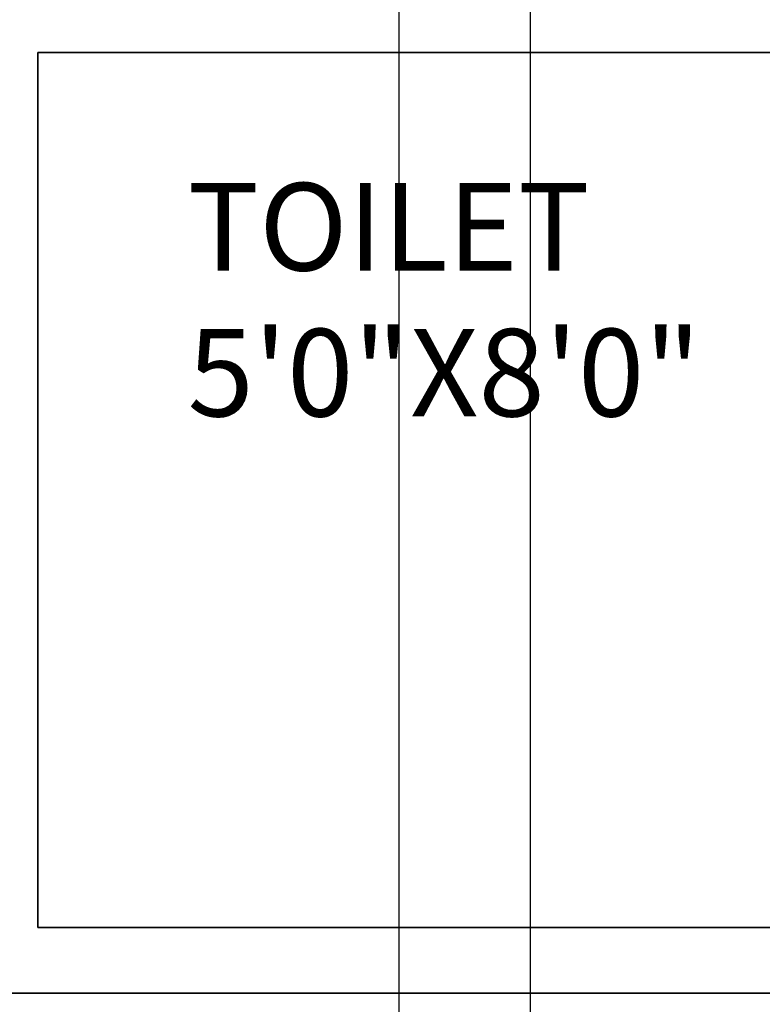
# Model space of a CAD drawing. Units: inches. Extents: x 1088 to 1703, y 668 to 1875.
# Tile 29 of 45: x 1489 to 1539, y 1539 to 1606. Entities that reach past the tile are written whole.
import ezdxf

# ---------------------------------------------------------------- set-up
doc = ezdxf.new("R2010")
doc.units = ezdxf.units.IN
for name, color, linetype, lineweight in [('A-ANNO-DIMS', 2, 'Continuous', 18), ('A-AREA-IDEN', 7, 'Continuous', 18), ('A-WALL', 7, 'Continuous', 35)]:
    doc.layers.add(name, color=color, linetype=linetype, lineweight=lineweight)
doc.styles.get("Standard").update_dxf_attribs({"font": 'arial.ttf'})
doc.dimstyles.get("Standard").update_dxf_attribs({"dimtxt": 0.18, "dimasz": 0.18, "dimexe": 0.18, "dimexo": 0.0625, "dimgap": 0.09, "dimtad": 0, "dimtih": 1, "dimtoh": 1, "dimdec": 4, "dimzin": 0, "dimdsep": 46, "dimtxsty": 'Standard', "dimcen": 0.09, "dimadec": 0, "dimazin": 0, "dimtfac": 1, "dimtdec": 4, "dimtofl": 0, "dimtmove": 0, "dimatfit": 3, "dimfxl": 1, "dimtolj": 1, "dimtzin": 0, "dimarcsym": 0})

# ---------------------------------------------------------------- blocks, each defined once
blk = doc.blocks.new('*D33')
at = {"layer": 'A-ANNO-DIMS', "color": 0, "lineweight": -2, "transparency": 16777216}
for p, q in [((1514.595, 1355.648), (1514.595, 1857.788)), ((1523.595, 1331.121), (1523.595, 1857.788)), ((1514.775, 1857.608), (1518.946, 1857.608)), ((1523.415, 1857.608), (1519.244, 1857.608))]:
    blk.add_line(p, q, dxfattribs=at)
at = {"layer": 'A-ANNO-DIMS', "color": 0, "transparency": 16777216}
for points in [[(1514.775, 1857.638), (1514.775, 1857.578), (1514.595, 1857.608)], [(1523.415, 1857.638), (1523.415, 1857.578), (1523.595, 1857.608)]]:
    blk.add_solid(points, dxfattribs=at)
at = {"layer": 'Defpoints', "color": 0, "transparency": 16777216}
for p in [(1523.595, 1857.608), (1514.595, 1355.585), (1523.595, 1331.058)]:
    blk.add_point(p, dxfattribs=at)
at = {"layer": 'A-ANNO-DIMS', "color": 0, "transparency": 16777216, "insert": (1519.095, 1857.608), "char_height": 0.18, "attachment_point": 5}
blk.add_mtext('\\A1;9', dxfattribs=at)

msp = doc.modelspace()

# ---------------------------------------------------------------- linework, layer by layer
at = {"layer": 'A-WALL'}
for p, q in [((1489.845, 1604.058), (1585.845, 1604.058)), ((1489.845, 1544.058), (1489.845, 1604.058)), ((1562.251, 1544.058), (1489.845, 1544.058)), ((1485.345, 1539.558), (1560.928, 1539.558))]:
    msp.add_line(p, q, dxfattribs=at)

# ---------------------------------------------------------------- texts
at = {"layer": 'A-AREA-IDEN', "insert": (1500.094, 1595.111), "char_height": 6, "attachment_point": 1}
msp.add_mtext_dynamic_manual_height_columns('TOILET\\P5\'0"X8\'0"', width=103.47088, gutter_width=12.5, heights=[0], dxfattribs=at)

# ---------------------------------------------------------------- dimensions: what is measured, and where the dimension line sits
at = {"layer": 'A-ANNO-DIMS'}
dim = msp.add_linear_dim(base=(1523.595, 1857.608), p1=(1514.595, 1355.585), p2=(1523.595, 1331.058), dimstyle='Standard', override={"dimdec": 0, "dimlfac": 1, "dimrnd": 0, "dimzin": 0, "dimdsep": 46, "dimlunit": 2}, dxfattribs=at)
dim.commit()
dim.dimension.update_dxf_attribs({"geometry": '*D33', "text_midpoint": (1519.095, 1857.608)})

doc.saveas('drawing.dxf')
